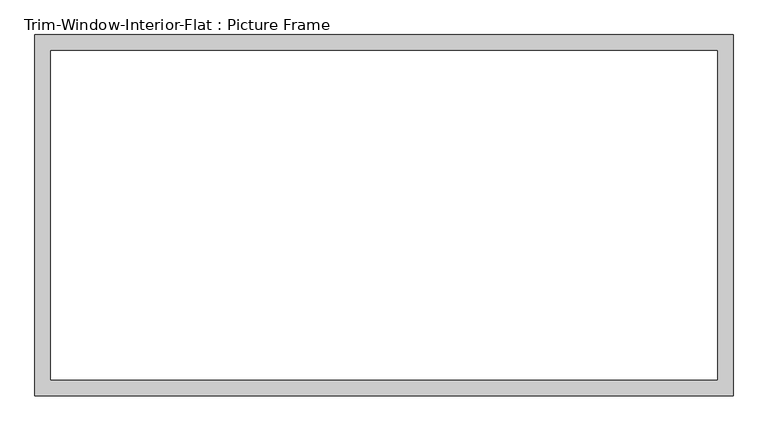
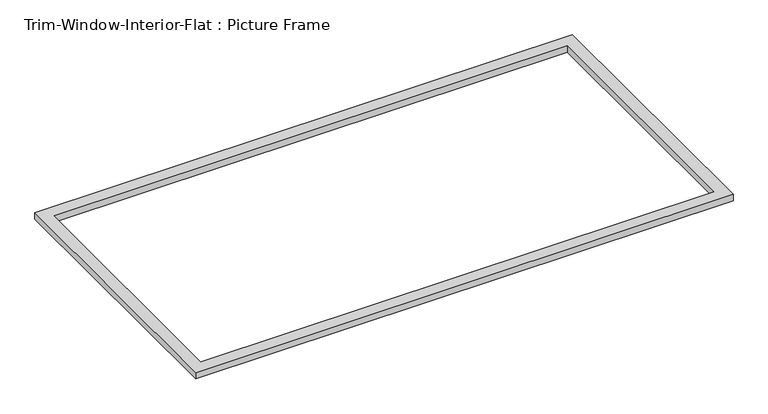
"""IFC4 building model written with IfcOpenShell, lengths in millimetres: proxy geometry, Trim-Window-Interior-Flat : Picture Frame."""

from ifc_helpers import new_model, si_unit, origin, origin_with_axes, place, context, project, spatial, polyline, outline, extrude, source, transform, mapped, element, save


def trim_window_interior_flat_picture_frame_d03d3773(model_context):
    return source(origin(), model_context, "Body", "SweptSolid", [
        extrude(outline(polyline([(1263.65, 44.45), (1263.65, -1263.65), (-1263.65, -1263.65), (-1263.65, 44.45), (1263.65, 44.45)]), holes=[polyline([(1206.5, -12.7), (-1206.5, -12.7), (-1206.5, -1206.5), (1206.5, -1206.5), (1206.5, -12.7)])]), origin_with_axes(), (0.0, 0.0, 1.0), 31.75),
    ])


if __name__ == "__main__":
    model = new_model("IFC4")
    model_context = context("Model", 3, world=origin())
    ifc_project = project(units=[si_unit("LENGTHUNIT", "METRE", prefix="MILLI")], contexts=[model_context])
    site = spatial("IfcSite", under=ifc_project)
    building = spatial("IfcBuilding", under=site)
    placement = place(None, origin())
    trim_window_interior_flat_picture_frame_shape = trim_window_interior_flat_picture_frame_d03d3773(model_context)
    element("IfcBuildingElementProxy", 1, Name="Trim-Window-Interior-Flat : Picture Frame", ObjectType="Trim-Window-Interior-Flat : Picture Frame", at=placement, inside=building, context=model_context, shape_type="MappedRepresentation", body=[
        mapped(trim_window_interior_flat_picture_frame_shape, transform((0.0, 0.0, 0.0), x_axis=(1.0, 0.0, 0.0), y_axis=(0.0, 1.0, 0.0), z_axis=(0.0, 0.0, 1.0))),
    ])
    save(model, "model.ifc")

# Revit data of these elements
# Type "Trim-Window-Interior-Flat : Picture Frame"
#   Trim Thickness_Picture Frame = 0' - 1 1/4"
#   Trim Width = 0' - 2 1/4"
#   Trim Thickness_with Sill = 0' - 0 3/4"
#   Sill Thickness = 0' - 1 1/4"
#   Opening Width [instance default] = 2' - 0"
#   Opening Height [instance default] = 3' - 0"
#   Default Elevation = 4' - 0"
#   Sill = no
#   Picture Frame = yes
#   Trim Material [instance default] = none
# Element 1 (IfcBuildingElementProxy, "Trim-Window-Interior-Flat : Picture Frame")
#   Opening Width = 8' - 0"
#   Opening Height = 4' - 0"
#   Trim Material = Wood - Stained
#   Materials on its faces: "Wood - Stained"
# Materials
#   "Wood - Stained": class "Wood", colour RGB 224 178 126, transparency 0, Cost = 0
